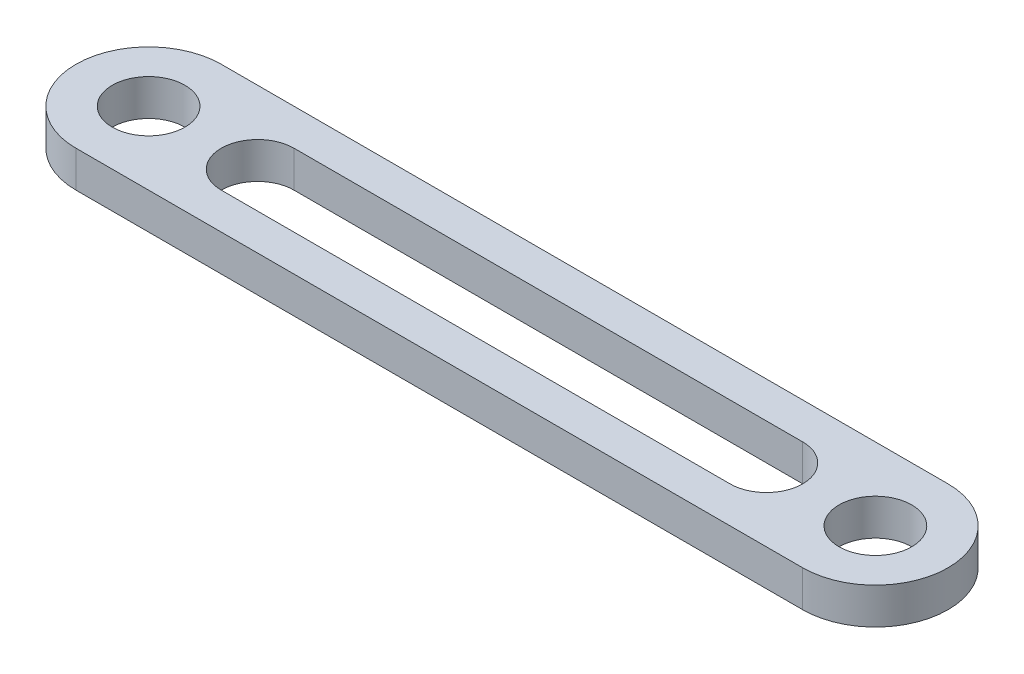
from build123d import *

# Parameters (mm, degrees)
LINK_PROFILE_SKETCH_R = 5
LINK_PLATE_5MM_DEPTH  = 5


with BuildPart() as part:
    # Link Profile Sketch → Link Plate 5mm (new body)
    with BuildSketch(Plane(origin=(0, 0, 0), x_dir=(1, 0, 0), z_dir=(0, 1, 0))):
        with BuildLine():
            Line((-50, 10), (50, 10))
            ThreePointArc((50, 10), (60, 0), (50, -10))
            Line((50, -10), (-50, -10))
            ThreePointArc((-50, -10), (-60, 0), (-50, 10))
        make_face()
        with Locations(Location((-50, 0, 0), (0, 0, 270))):
            Circle(LINK_PROFILE_SKETCH_R, mode=Mode.SUBTRACT)
        with Locations(Location((50, 0, 0), (0, 0, 270))):
            Circle(LINK_PROFILE_SKETCH_R, mode=Mode.SUBTRACT)
        with BuildLine():
            Line((-35, 5), (35, 5))
            ThreePointArc((35, 5), (40, 0), (35, -5))
            Line((35, -5), (-35, -5))
            ThreePointArc((-35, -5), (-40, 0), (-35, 5))
        make_face(mode=Mode.SUBTRACT)
    extrude(amount=LINK_PLATE_5MM_DEPTH)


solid = part.part
